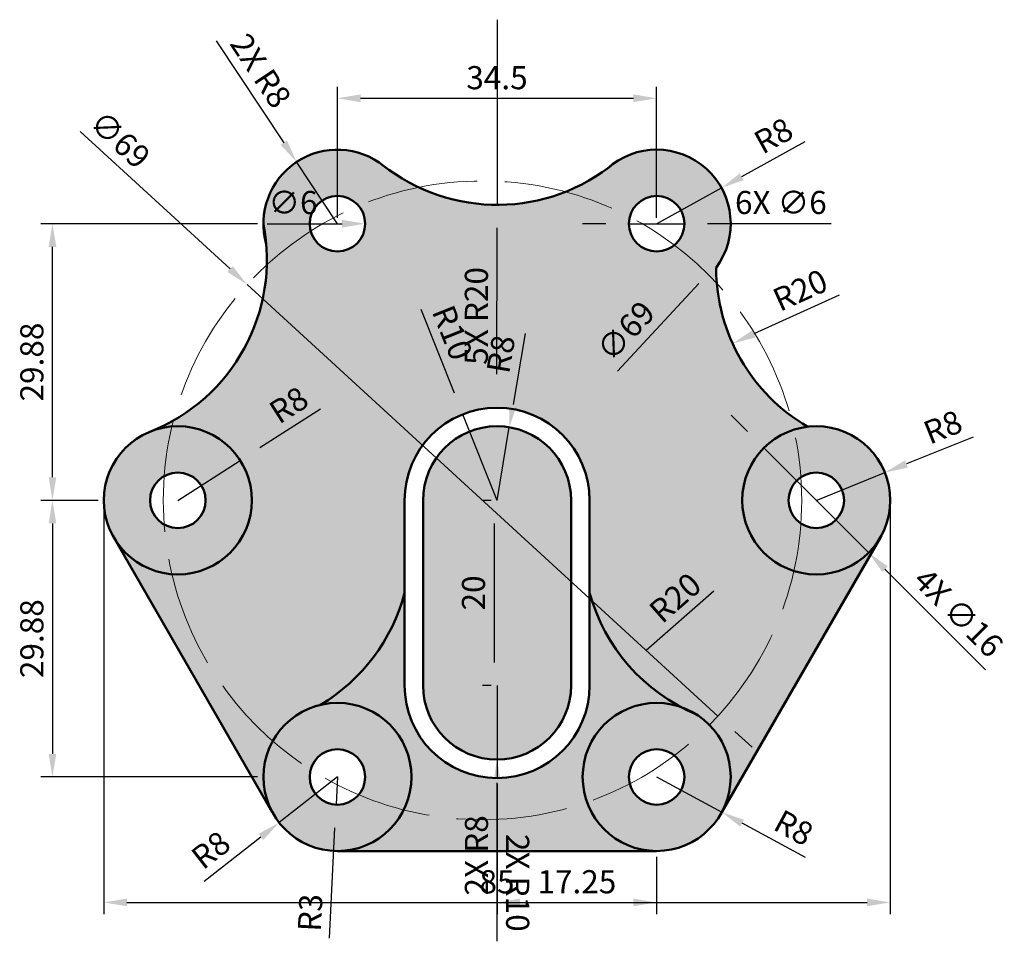
# Model space of a CAD drawing. Units: millimetres. Extents: x 3056 to 3163, y 1664 to 1764.
import ezdxf

# ---------------------------------------------------------------- set-up
doc = ezdxf.new("R2010")
doc.units = ezdxf.units.MM
doc.linetypes.add('ACAD_ISO02W100', pattern=[15, 12, -3])
for name, color, linetype, lineweight in [('M-CONS', 8, 'ACAD_ISO02W100', 18), ('M-DIMS', 2, 'Continuous', 25), ('M-HATC', 252, 'Continuous', 18), ('M-OUTL', 7, 'Continuous', 50)]:
    doc.layers.add(name, color=color, linetype=linetype, lineweight=lineweight)
doc.styles.get("Standard").update_dxf_attribs({"font": 'arial.ttf'})
doc.dimstyles.new('ISO-25', dxfattribs={"dimtxt": 2.5, "dimasz": 2.5, "dimexe": 1.25, "dimexo": 0.625, "dimtad": 1, "dimtxsty": 'Standard', "dimcen": 2.5, "dimadec": 0, "dimazin": 0, "dimtfac": 1, "dimtmove": 0, "dimatfit": 3, "dimfxl": 1, "dimarcsym": 0})

# ---------------------------------------------------------------- blocks, each defined once
blk = doc.blocks.new('*D1')
at = {"layer": 'Defpoints', "color": 0, "transparency": 16777216}
for p in [(3131.59, 1737.12), (3084.57, 1686.62)]:
    blk.add_point(p, dxfattribs=at)
at = {"layer": 'M-DIMS', "color": 0, "lineweight": -2, "transparency": 16777216}
blk.add_line((3121.1, 1725.84), (3129.89, 1735.29), dxfattribs=at)
at = {"layer": 'M-DIMS', "color": 0, "transparency": 16777216}
blk.add_solid([(3129.59, 1735.57), (3130.2, 1735.01), (3131.59, 1737.12)], dxfattribs=at)
at = {"layer": 'M-DIMS', "color": 0, "transparency": 16777216, "insert": (3122.23, 1729.95), "char_height": 2.5, "attachment_point": 5, "rotation": 47.0416}
blk.add_mtext('∅69', dxfattribs=at)
blk = doc.blocks.new('*D2')
at = {"layer": 'Defpoints', "color": 0, "transparency": 16777216}
for p in [(3087.83, 1741.75), (3093.83, 1741.75)]:
    blk.add_point(p, dxfattribs=at)
at = {"layer": 'M-DIMS', "color": 0, "lineweight": -2, "transparency": 16777216}
blk.add_line((3083.23, 1741.75), (3091.33, 1741.75), dxfattribs=at)
at = {"layer": 'M-DIMS', "color": 0, "transparency": 16777216}
blk.add_solid([(3091.33, 1742.17), (3091.33, 1741.33), (3093.83, 1741.75)], dxfattribs=at)
at = {"layer": 'M-DIMS', "color": 0, "transparency": 16777216, "insert": (3086.03, 1743.72), "char_height": 2.5, "attachment_point": 5}
blk.add_mtext('∅6', dxfattribs=at)
blk = doc.blocks.new('*D3')
at = {"layer": 'Defpoints', "color": 0, "transparency": 16777216}
for p in [(3132.34, 1745.62), (3125.33, 1741.75)]:
    blk.add_point(p, dxfattribs=at)
at = {"layer": 'M-DIMS', "color": 0, "lineweight": -2, "transparency": 16777216}
for p, q in [((3141.34, 1750.59), (3134.52, 1746.83)), ((3125.33, 1741.75), (3132.34, 1745.62))]:
    blk.add_line(p, q, dxfattribs=at)
at = {"layer": 'M-DIMS', "color": 0, "transparency": 16777216}
blk.add_solid([(3134.32, 1747.19), (3134.73, 1746.46), (3132.34, 1745.62)], dxfattribs=at)
at = {"layer": 'M-DIMS', "color": 0, "transparency": 16777216, "insert": (3138.11, 1750.98), "char_height": 2.5, "attachment_point": 5, "rotation": 28.9236}
blk.add_mtext('R8', dxfattribs=at)
blk = doc.blocks.new('*D4')
at = {"layer": 'Defpoints', "color": 0, "transparency": 16777216}
for p in [(3151.75, 1737.08), (3133.54, 1728.81)]:
    blk.add_point(p, dxfattribs=at)
at = {"layer": 'M-DIMS', "color": 0, "lineweight": -2, "transparency": 16777216}
blk.add_line((3145.05, 1734.04), (3135.82, 1729.85), dxfattribs=at)
at = {"layer": 'M-DIMS', "color": 0, "transparency": 16777216}
blk.add_solid([(3135.65, 1730.22), (3135.99, 1729.47), (3133.54, 1728.81)], dxfattribs=at)
at = {"layer": 'M-DIMS', "color": 0, "transparency": 16777216, "insert": (3140.98, 1734.28), "char_height": 2.5, "attachment_point": 5, "rotation": 24.4299}
blk.add_mtext('R20', dxfattribs=at)
blk = doc.blocks.new('*D5')
at = {"layer": 'Defpoints', "color": 0, "transparency": 16777216}
for p in [(3109.41, 1719.76), (3108.08, 1711.87)]:
    blk.add_point(p, dxfattribs=at)
at = {"layer": 'M-DIMS', "color": 0, "lineweight": -2, "transparency": 16777216}
for p, q in [((3111.12, 1729.9), (3109.83, 1722.23)), ((3108.08, 1711.87), (3109.41, 1719.76))]:
    blk.add_line(p, q, dxfattribs=at)
at = {"layer": 'M-DIMS', "color": 0, "transparency": 16777216}
blk.add_solid([(3109.42, 1722.29), (3110.24, 1722.16), (3109.41, 1719.76)], dxfattribs=at)
at = {"layer": 'M-DIMS', "color": 0, "transparency": 16777216, "insert": (3108.81, 1727.61), "char_height": 2.5, "attachment_point": 5, "rotation": 80.4313}
blk.add_mtext('R8', dxfattribs=at)
blk = doc.blocks.new('*D6')
at = {"layer": 'Defpoints', "color": 0, "transparency": 16777216}
for p in [(3104.38, 1721.16), (3108.08, 1711.87)]:
    blk.add_point(p, dxfattribs=at)
at = {"layer": 'M-DIMS', "color": 0, "lineweight": -2, "transparency": 16777216}
for p, q in [((3099.86, 1732.51), (3103.45, 1723.48)), ((3108.08, 1711.87), (3104.38, 1721.16))]:
    blk.add_line(p, q, dxfattribs=at)
at = {"layer": 'M-DIMS', "color": 0, "transparency": 16777216}
blk.add_solid([(3103.84, 1723.64), (3103.07, 1723.33), (3104.38, 1721.16)], dxfattribs=at)
at = {"layer": 'M-DIMS', "color": 0, "transparency": 16777216, "insert": (3102.96, 1729.86), "char_height": 2.5, "attachment_point": 5, "rotation": 291.7372}
blk.add_mtext('R10', dxfattribs=at)
blk = doc.blocks.new('*D7')
at = {"layer": 'Defpoints', "color": 0, "transparency": 16777216}
for p in [(3137.36, 1707.2), (3122.33, 1694)]:
    blk.add_point(p, dxfattribs=at)
at = {"layer": 'M-DIMS', "color": 0, "lineweight": -2, "transparency": 16777216}
blk.add_line((3131.51, 1702.06), (3124.21, 1695.65), dxfattribs=at)
at = {"layer": 'M-DIMS', "color": 0, "transparency": 16777216}
blk.add_solid([(3123.93, 1695.97), (3124.48, 1695.34), (3122.33, 1694)], dxfattribs=at)
at = {"layer": 'M-DIMS', "color": 0, "transparency": 16777216, "insert": (3127.55, 1701.11), "char_height": 2.5, "attachment_point": 5, "rotation": 41.2749}
blk.add_mtext('R20', dxfattribs=at)
blk = doc.blocks.new('*D8')
at = {"layer": 'Defpoints', "color": 0, "transparency": 16777216}
for p in [(3090.83, 1681.99), (3090.69, 1679)]:
    blk.add_point(p, dxfattribs=at)
at = {"layer": 'M-DIMS', "color": 0, "lineweight": -2, "transparency": 16777216}
for p, q in [((3090.83, 1681.99), (3090.69, 1679)), ((3089.98, 1664.59), (3090.56, 1676.5))]:
    blk.add_line(p, q, dxfattribs=at)
at = {"layer": 'M-DIMS', "color": 0, "transparency": 16777216}
blk.add_solid([(3090.15, 1676.52), (3090.98, 1676.48), (3090.69, 1679)], dxfattribs=at)
at = {"layer": 'M-DIMS', "color": 0, "transparency": 16777216, "insert": (3088.21, 1667.32), "char_height": 2.5, "attachment_point": 5, "rotation": 87.1851}
blk.add_mtext('R3', dxfattribs=at)
blk = doc.blocks.new('*D9')
at = {"layer": 'Defpoints', "color": 0, "transparency": 16777216}
for p in [(3090.83, 1681.99), (3084.53, 1677.06)]:
    blk.add_point(p, dxfattribs=at)
at = {"layer": 'M-DIMS', "color": 0, "lineweight": -2, "transparency": 16777216}
for p, q in [((3090.83, 1681.99), (3084.53, 1677.06)), ((3076.44, 1670.72), (3082.57, 1675.52))]:
    blk.add_line(p, q, dxfattribs=at)
at = {"layer": 'M-DIMS', "color": 0, "transparency": 16777216}
blk.add_solid([(3082.31, 1675.85), (3082.82, 1675.19), (3084.53, 1677.06)], dxfattribs=at)
at = {"layer": 'M-DIMS', "color": 0, "transparency": 16777216, "insert": (3077.34, 1673.85), "char_height": 2.5, "attachment_point": 5, "rotation": 38.0577}
blk.add_mtext('R8', dxfattribs=at)
blk = doc.blocks.new('*D10')
at = {"layer": 'Defpoints', "color": 0, "transparency": 16777216}
for p in [(3125.33, 1681.99), (3132.37, 1678.19)]:
    blk.add_point(p, dxfattribs=at)
at = {"layer": 'M-DIMS', "color": 0, "lineweight": -2, "transparency": 16777216}
for p, q in [((3125.33, 1681.99), (3132.37, 1678.19)), ((3141.42, 1673.3), (3134.57, 1677))]:
    blk.add_line(p, q, dxfattribs=at)
at = {"layer": 'M-DIMS', "color": 0, "transparency": 16777216}
blk.add_solid([(3134.77, 1677.37), (3134.37, 1676.63), (3132.37, 1678.19)], dxfattribs=at)
at = {"layer": 'M-DIMS', "color": 0, "transparency": 16777216, "insert": (3140, 1676.23), "char_height": 2.5, "attachment_point": 5, "rotation": 331.5993}
blk.add_mtext('R8', dxfattribs=at)
blk = doc.blocks.new('*D11')
at = {"layer": 'Defpoints', "color": 0, "transparency": 16777216}
for p in [(3150, 1714.87), (3142.58, 1711.87)]:
    blk.add_point(p, dxfattribs=at)
at = {"layer": 'M-DIMS', "color": 0, "lineweight": -2, "transparency": 16777216}
for p, q in [((3159.54, 1718.71), (3152.32, 1715.8)), ((3142.58, 1711.87), (3150, 1714.87))]:
    blk.add_line(p, q, dxfattribs=at)
at = {"layer": 'M-DIMS', "color": 0, "transparency": 16777216}
blk.add_solid([(3152.17, 1716.19), (3152.48, 1715.41), (3150, 1714.87)], dxfattribs=at)
at = {"layer": 'M-DIMS', "color": 0, "transparency": 16777216, "insert": (3156.38, 1719.49), "char_height": 2.5, "attachment_point": 5, "rotation": 21.9727}
blk.add_mtext('R8', dxfattribs=at)
blk = doc.blocks.new('*D12')
at = {"layer": 'Defpoints', "color": 0, "transparency": 16777216}
for p in [(3080.33, 1716.18), (3073.58, 1711.87)]:
    blk.add_point(p, dxfattribs=at)
at = {"layer": 'M-DIMS', "color": 0, "lineweight": -2, "transparency": 16777216}
for p, q in [((3088.99, 1721.72), (3082.43, 1717.53)), ((3073.58, 1711.87), (3080.33, 1716.18))]:
    blk.add_line(p, q, dxfattribs=at)
at = {"layer": 'M-DIMS', "color": 0, "transparency": 16777216}
blk.add_solid([(3082.21, 1717.88), (3082.66, 1717.17), (3080.33, 1716.18)], dxfattribs=at)
at = {"layer": 'M-DIMS', "color": 0, "transparency": 16777216, "insert": (3085.74, 1721.9), "char_height": 2.5, "attachment_point": 5, "rotation": 32.5786}
blk.add_mtext('R8', dxfattribs=at)
blk = doc.blocks.new('*D13')
at = {"layer": 'Defpoints', "color": 0, "transparency": 16777216}
for p in [(3108.08, 1711.87), (3107.76, 1691.87), (3108.08, 1691.87)]:
    blk.add_point(p, dxfattribs=at)
at = {"layer": 'M-DIMS', "color": 0, "lineweight": -2, "transparency": 16777216}
for p, q in [((3107.46, 1711.87), (3106.51, 1711.87)), ((3107.76, 1709.37), (3107.76, 1694.37)), ((3107.46, 1691.87), (3106.51, 1691.87))]:
    blk.add_line(p, q, dxfattribs=at)
at = {"layer": 'M-DIMS', "color": 0, "transparency": 16777216}
for points in [[(3107.35, 1709.37), (3108.18, 1709.37), (3107.76, 1711.87)], [(3107.35, 1694.37), (3108.18, 1694.37), (3107.76, 1691.87)]]:
    blk.add_solid(points, dxfattribs=at)
at = {"layer": 'M-DIMS', "color": 0, "transparency": 16777216, "insert": (3105.86, 1701.87), "char_height": 2.5, "attachment_point": 5, "rotation": 90}
blk.add_mtext('20', dxfattribs=at)
blk = doc.blocks.new('MOUNTING-BOSS-16-BORE-6')
for radius in [8, 3]:
    blk.add_circle((8, 8), radius)
blk = doc.blocks.new('*D15')
at = {"layer": 'Defpoints', "color": 0, "transparency": 16777216}
for p in [(3065.58, 1711.87), (3150.58, 1711.87), (3150.58, 1668.44)]:
    blk.add_point(p, dxfattribs=at)
at = {"layer": 'M-DIMS', "color": 0, "lineweight": -2, "transparency": 16777216}
for p, q in [((3065.58, 1711.25), (3065.58, 1667.19)), ((3150.58, 1711.25), (3150.58, 1667.19)), ((3068.08, 1668.44), (3148.08, 1668.44))]:
    blk.add_line(p, q, dxfattribs=at)
at = {"layer": 'M-DIMS', "color": 0, "transparency": 16777216}
for points in [[(3068.08, 1668.86), (3068.08, 1668.03), (3065.58, 1668.44)], [(3148.08, 1668.86), (3148.08, 1668.03), (3150.58, 1668.44)]]:
    blk.add_solid(points, dxfattribs=at)
at = {"layer": 'M-DIMS', "color": 0, "transparency": 16777216, "insert": (3108.08, 1670.35), "char_height": 2.5, "attachment_point": 5}
blk.add_mtext('85', dxfattribs=at)
blk = doc.blocks.new('*D16')
at = {"layer": 'Defpoints', "color": 0, "transparency": 16777216}
for p in [(3125.33, 1755.3), (3090.83, 1741.75), (3125.33, 1741.75)]:
    blk.add_point(p, dxfattribs=at)
at = {"layer": 'M-DIMS', "color": 0, "lineweight": -2, "transparency": 16777216}
for p, q in [((3090.83, 1742.37), (3090.83, 1756.55)), ((3125.33, 1742.37), (3125.33, 1756.55)), ((3093.33, 1755.3), (3122.83, 1755.3))]:
    blk.add_line(p, q, dxfattribs=at)
at = {"layer": 'M-DIMS', "color": 0, "transparency": 16777216}
for points in [[(3093.33, 1755.72), (3093.33, 1754.88), (3090.83, 1755.3)], [(3122.83, 1755.72), (3122.83, 1754.88), (3125.33, 1755.3)]]:
    blk.add_solid(points, dxfattribs=at)
at = {"layer": 'M-DIMS', "color": 0, "transparency": 16777216, "insert": (3108.08, 1757.2), "char_height": 2.5, "attachment_point": 5}
blk.add_mtext('34.5', dxfattribs=at)
blk = doc.blocks.new('*D17')
at = {"layer": 'Defpoints', "color": 0, "transparency": 16777216}
for p in [(3108.08, 1681.87), (3125.33, 1673.99), (3125.33, 1668.44)]:
    blk.add_point(p, dxfattribs=at)
at = {"layer": 'M-DIMS', "color": 0, "lineweight": -2, "transparency": 16777216}
for p, q in [((3108.08, 1681.25), (3108.08, 1667.19)), ((3125.33, 1673.37), (3125.33, 1667.19)), ((3110.58, 1668.44), (3122.83, 1668.44))]:
    blk.add_line(p, q, dxfattribs=at)
at = {"layer": 'M-DIMS', "color": 0, "transparency": 16777216}
for points in [[(3110.58, 1668.86), (3110.58, 1668.03), (3108.08, 1668.44)], [(3122.83, 1668.86), (3122.83, 1668.03), (3125.33, 1668.44)]]:
    blk.add_solid(points, dxfattribs=at)
at = {"layer": 'M-DIMS', "color": 0, "transparency": 16777216, "insert": (3116.71, 1670.35), "char_height": 2.5, "attachment_point": 5}
blk.add_mtext('17.25', dxfattribs=at)
blk = doc.blocks.new('*D18')
at = {"layer": 'Defpoints', "color": 0, "transparency": 16777216}
for p in [(3060.03, 1741.75), (3082.83, 1741.75), (3065.58, 1711.87)]:
    blk.add_point(p, dxfattribs=at)
at = {"layer": 'M-DIMS', "color": 0, "lineweight": -2, "transparency": 16777216}
for p, q in [((3082.21, 1741.75), (3058.78, 1741.75)), ((3060.03, 1714.37), (3060.03, 1739.25)), ((3064.96, 1711.87), (3058.78, 1711.87))]:
    blk.add_line(p, q, dxfattribs=at)
at = {"layer": 'M-DIMS', "color": 0, "transparency": 16777216}
for points in [[(3059.62, 1739.25), (3060.45, 1739.25), (3060.03, 1741.75)], [(3059.62, 1714.37), (3060.45, 1714.37), (3060.03, 1711.87)]]:
    blk.add_solid(points, dxfattribs=at)
at = {"layer": 'M-DIMS', "color": 0, "transparency": 16777216, "insert": (3058.13, 1726.81), "char_height": 2.5, "attachment_point": 5, "rotation": 90}
blk.add_mtext('29.88', dxfattribs=at)
blk = doc.blocks.new('*D19')
at = {"layer": 'Defpoints', "color": 0, "transparency": 16777216}
for p in [(3065.58, 1711.87), (3060.03, 1681.99), (3082.83, 1681.99)]:
    blk.add_point(p, dxfattribs=at)
at = {"layer": 'M-DIMS', "color": 0, "lineweight": -2, "transparency": 16777216}
for p, q in [((3064.96, 1711.87), (3058.78, 1711.87)), ((3060.03, 1709.37), (3060.03, 1684.49)), ((3082.21, 1681.99), (3058.78, 1681.99))]:
    blk.add_line(p, q, dxfattribs=at)
at = {"layer": 'M-DIMS', "color": 0, "transparency": 16777216}
for points in [[(3059.62, 1709.37), (3060.45, 1709.37), (3060.03, 1711.87)], [(3059.62, 1684.49), (3060.45, 1684.49), (3060.03, 1681.99)]]:
    blk.add_solid(points, dxfattribs=at)
at = {"layer": 'M-DIMS', "color": 0, "transparency": 16777216, "insert": (3058.13, 1696.93), "char_height": 2.5, "attachment_point": 5, "rotation": 90}
blk.add_mtext('29.88', dxfattribs=at)
blk = doc.blocks.new('*D20')
at = {"layer": 'Defpoints', "color": 0, "transparency": 16777216}
for p in [(3122.33, 1741.75), (3128.33, 1741.75)]:
    blk.add_point(p, dxfattribs=at)
at = {"layer": 'M-DIMS', "color": 0, "lineweight": -2, "transparency": 16777216}
for p, q in [((3119.83, 1741.75), (3117.33, 1741.75)), ((3122.33, 1741.75), (3128.33, 1741.75)), ((3144.19, 1741.75), (3130.83, 1741.75))]:
    blk.add_line(p, q, dxfattribs=at)
at = {"layer": 'M-DIMS', "color": 0, "transparency": 16777216}
for points in [[(3119.83, 1742.17), (3119.83, 1741.33), (3122.33, 1741.75)], [(3130.83, 1742.17), (3130.83, 1741.33), (3128.33, 1741.75)]]:
    blk.add_solid(points, dxfattribs=at)
at = {"layer": 'M-DIMS', "color": 0, "transparency": 16777216, "insert": (3138.76, 1743.72), "char_height": 2.5, "attachment_point": 5, "rotation": 0.0066}
blk.add_mtext('6X ∅6', dxfattribs=at)
blk = doc.blocks.new('*D21')
at = {"layer": 'Defpoints', "color": 0, "transparency": 16777216}
for p in [(3136.93, 1717.53), (3148.24, 1706.22)]:
    blk.add_point(p, dxfattribs=at)
at = {"layer": 'M-DIMS', "color": 0, "lineweight": -2, "transparency": 16777216}
for p, q in [((3135.16, 1719.3), (3133.39, 1721.06)), ((3136.93, 1717.53), (3148.24, 1706.22)), ((3160.89, 1693.57), (3150.01, 1704.45))]:
    blk.add_line(p, q, dxfattribs=at)
at = {"layer": 'M-DIMS', "color": 0, "transparency": 16777216}
for points in [[(3135.45, 1719.59), (3134.86, 1719), (3136.93, 1717.53)], [(3150.3, 1704.74), (3149.71, 1704.15), (3148.24, 1706.22)]]:
    blk.add_solid(points, dxfattribs=at)
at = {"layer": 'M-DIMS', "color": 0, "transparency": 16777216, "insert": (3157.73, 1699.52), "char_height": 2.5, "attachment_point": 5, "rotation": 315.0013}
blk.add_mtext('4X ∅16', dxfattribs=at)
blk = doc.blocks.new('*D22')
at = {"layer": 'Defpoints', "color": 0, "transparency": 16777216}
for p in [(3081.07, 1735.17), (3131.96, 1688.57)]:
    blk.add_point(p, dxfattribs=at)
at = {"layer": 'M-DIMS', "color": 0, "lineweight": -2, "transparency": 16777216}
for p, q in [((3063.02, 1751.7), (3079.23, 1736.86)), ((3131.96, 1688.57), (3081.07, 1735.17)), ((3133.8, 1686.89), (3135.65, 1685.2))]:
    blk.add_line(p, q, dxfattribs=at)
at = {"layer": 'M-DIMS', "color": 0, "transparency": 16777216}
for points in [[(3079.51, 1737.17), (3078.94, 1736.55), (3081.07, 1735.17)], [(3134.08, 1687.19), (3133.52, 1686.58), (3131.96, 1688.57)]]:
    blk.add_solid(points, dxfattribs=at)
at = {"layer": 'M-DIMS', "color": 0, "transparency": 16777216, "insert": (3067.13, 1750.6), "char_height": 2.5, "attachment_point": 5, "rotation": 317.5212}
blk.add_mtext('∅69', dxfattribs=at)
blk = doc.blocks.new('*D23')
at = {"layer": 'Defpoints', "color": 0, "transparency": 16777216}
for p in [(3108.11, 1763.79), (3108.08, 1743.79)]:
    blk.add_point(p, dxfattribs=at)
at = {"layer": 'M-DIMS', "color": 0, "lineweight": -2, "transparency": 16777216}
for p, q in [((3108.11, 1763.79), (3108.08, 1743.79)), ((3108.06, 1725.49), (3108.08, 1741.29))]:
    blk.add_line(p, q, dxfattribs=at)
at = {"layer": 'M-DIMS', "color": 0, "transparency": 16777216}
blk.add_solid([(3107.66, 1741.29), (3108.5, 1741.29), (3108.08, 1743.79)], dxfattribs=at)
at = {"layer": 'M-DIMS', "color": 0, "transparency": 16777216, "insert": (3106.17, 1731.79), "char_height": 2.5, "attachment_point": 5, "rotation": 89.9384}
blk.add_mtext('5X R20', dxfattribs=at)
blk = doc.blocks.new('*D24')
at = {"layer": 'Defpoints', "color": 0, "transparency": 16777216}
for p in [(3108.08, 1691.87), (3108.08, 1681.87)]:
    blk.add_point(p, dxfattribs=at)
at = {"layer": 'M-DIMS', "color": 0, "lineweight": -2, "transparency": 16777216}
for p, q in [((3108.08, 1691.87), (3108.08, 1681.87)), ((3108.08, 1664.24), (3108.08, 1679.37))]:
    blk.add_line(p, q, dxfattribs=at)
at = {"layer": 'M-DIMS', "color": 0, "transparency": 16777216}
blk.add_solid([(3108.5, 1679.37), (3107.67, 1679.37), (3108.08, 1681.87)], dxfattribs=at)
at = {"layer": 'M-DIMS', "color": 0, "transparency": 16777216, "insert": (3109.99, 1670.56), "char_height": 2.5, "attachment_point": 5, "rotation": 270.0002}
blk.add_mtext('2X R10', dxfattribs=at)
blk = doc.blocks.new('*D25')
at = {"layer": 'Defpoints', "color": 0, "transparency": 16777216}
for p in [(3086.42, 1748.42), (3090.83, 1741.75)]:
    blk.add_point(p, dxfattribs=at)
at = {"layer": 'M-DIMS', "color": 0, "lineweight": -2, "transparency": 16777216}
for p, q in [((3077.74, 1761.51), (3085.03, 1750.5)), ((3090.83, 1741.75), (3086.42, 1748.42))]:
    blk.add_line(p, q, dxfattribs=at)
at = {"layer": 'M-DIMS', "color": 0, "transparency": 16777216}
blk.add_solid([(3085.38, 1750.73), (3084.69, 1750.27), (3086.42, 1748.42)], dxfattribs=at)
at = {"layer": 'M-DIMS', "color": 0, "transparency": 16777216, "insert": (3082.28, 1758.1), "char_height": 2.5, "attachment_point": 5, "rotation": 303.5276}
blk.add_mtext('2X R8', dxfattribs=at)
blk = doc.blocks.new('*D26')
at = {"layer": 'Defpoints', "color": 0, "transparency": 16777216}
for p in [(3108.08, 1691.87), (3108.08, 1683.87)]:
    blk.add_point(p, dxfattribs=at)
at = {"layer": 'M-DIMS', "color": 0, "lineweight": -2, "transparency": 16777216}
for p, q in [((3108.08, 1691.87), (3108.08, 1683.87)), ((3108.08, 1668.17), (3108.08, 1681.37))]:
    blk.add_line(p, q, dxfattribs=at)
at = {"layer": 'M-DIMS', "color": 0, "transparency": 16777216}
blk.add_solid([(3107.67, 1681.37), (3108.5, 1681.37), (3108.08, 1683.87)], dxfattribs=at)
at = {"layer": 'M-DIMS', "color": 0, "transparency": 16777216, "insert": (3106.18, 1673.52), "char_height": 2.5, "attachment_point": 5, "rotation": 90}
blk.add_mtext('2X R8', dxfattribs=at)

msp = doc.modelspace()

# ---------------------------------------------------------------- hatches: boundary and pattern name
at = {"layer": 'M-HATC'}
h = msp.add_hatch(color=256, dxfattribs=at)
h.set_gradient(color1=(255, 255, 255), color2=(0, 255, 255), tint=1, name='INVSPHERICAL')
h.paths.add_polyline_path([(3131.752, 1736.973, 0.8439134), (3120.862, 1748.383, -0.3543215), (3095.679, 1748.115, 0.6204861), (3082.834, 1741.75, -0.3599737), (3070.694, 1719.331, -0.5271202), (3081.584, 1711.872, -0.7672909), (3066.656, 1707.871), (3083.797, 1678.189, -0.1245598), (3082.834, 1681.994, -0.3481695), (3089.005, 1689.782, 0.1962669), (3098.084, 1701.872), (3098.084, 1711.872, -1), (3118.084, 1711.872), (3118.084, 1701.872, 0.2053969), (3127.933, 1689.56, -0.3203024), (3133.334, 1681.994, -0.1245598), (3132.371, 1678.189), (3149.512, 1707.871, -0.7672909), (3134.584, 1711.872, -0.3805737), (3141.656, 1719.818, -0.265009)])
h.paths.add_polyline_path([(3087.834, 1741.75, -1), (3093.834, 1741.75, -1)], flags=16)
h.paths.add_polyline_path([(3122.334, 1741.75, -1), (3128.334, 1741.75, -1)], flags=16)
h.paths.add_polyline_path([(3121.467, 1725.306), (3126.817, 1731.051), (3123.047, 1734.562), (3117.696, 1728.816)], flags=24)
h.paths.add_polyline_path([(3083.085, 1741.11), (3088.994, 1741.11), (3088.994, 1746.262), (3083.085, 1746.262)], flags=24)
h.paths.add_polyline_path([(3110.887, 1724.304), (3111.837, 1729.939), (3106.757, 1730.796), (3105.807, 1725.161)], flags=24)
h.paths.add_polyline_path([(3099.107, 1732.504), (3101.943, 1725.392), (3106.728, 1727.3), (3103.892, 1734.412)], flags=24)
h.paths.add_polyline_path([(3126.342, 1696.598), (3132.097, 1701.649), (3128.698, 1705.52), (3122.944, 1700.469)], flags=24)
h.paths.add_polyline_path([(3084.683, 1718.136), (3089.498, 1721.213), (3086.724, 1725.554), (3081.909, 1722.477)], flags=24)
h = msp.add_hatch(color=256, dxfattribs=at)
h.set_gradient(color1=(255, 255, 255), color2=(248, 215, 49), tint=1, name='INVSPHERICAL')
h.paths.add_polyline_path([(3070.694, 1719.331, -0.0019683), (3070.548, 1719.273, 0.3042702), (3065.584, 1711.872, 1), (3081.584, 1711.872, 0.5271202)])
h.paths.add_polyline_path([(3076.584, 1711.872, -1), (3070.584, 1711.872, -1)], flags=16)
h.paths.add_polyline_path([(3082.834, 1681.994, 1), (3098.834, 1681.994, 1)])
h.paths.add_polyline_path([(3093.834, 1681.994, -1), (3087.834, 1681.994, -1)], flags=16)
h.paths.add_polyline_path([(3129.581, 1688.774, -0.0228354), (3127.933, 1689.56, 0.5148044), (3117.334, 1681.994, 1), (3133.334, 1681.994, 0.25832)])
h.paths.add_polyline_path([(3128.334, 1681.994, -1), (3122.334, 1681.994, -1)], flags=16)
h.paths.add_polyline_path([(3134.584, 1711.872, 1), (3150.584, 1711.872, 1)])
h.paths.add_polyline_path([(3145.584, 1711.872, -1), (3139.584, 1711.872, -1)], flags=16)
h = msp.add_hatch(color=256, dxfattribs=at)
h.set_gradient(color1=(255, 255, 255), color2=(255, 0, 255), tint=1, name='INVCYLINDER')
h.paths.add_polyline_path([(3100.084, 1711.872), (3100.084, 1691.872, 1), (3116.084, 1691.872), (3116.084, 1711.872, 1)])
h.paths.add_polyline_path([(3108.462, 1699.337), (3108.462, 1704.472), (3103.31, 1704.472), (3103.31, 1699.337)], flags=24)
h = msp.add_hatch(color=256, dxfattribs=at)
h.set_gradient(color1=(255, 255, 255), color2=(88, 186, 72), tint=1, name='HEMISPHERICAL')
h.paths.add_polyline_path([(3117.334, 1681.994, -0.5148044), (3127.933, 1689.56, -0.2053969), (3118.084, 1701.872), (3118.084, 1691.872, -1), (3098.084, 1691.872), (3098.084, 1701.872, -0.1962669), (3089.005, 1689.782, -0.483493), (3098.834, 1681.994, -0.4142136), (3090.834, 1673.994), (3125.334, 1673.994, -0.4142136)])

# ---------------------------------------------------------------- linework, layer by layer
at = {"layer": 'M-CONS'}
msp.add_circle((3106.514, 1711.872), 34.5, dxfattribs=at)
at = {"layer": 'M-OUTL'}
for p, q in [((3098.084, 1711.872), (3098.084, 1691.872)), ((3100.084, 1711.872), (3100.084, 1691.872)), ((3116.084, 1711.872), (3116.084, 1691.872)), ((3118.084, 1711.872), (3118.084, 1691.872)), ((3083.797, 1678.189), (3066.656, 1707.871)), ((3132.371, 1678.189), (3149.512, 1707.871)), ((3090.834, 1673.994), (3125.334, 1673.994))]:
    msp.add_line(p, q, dxfattribs=at)
for centre in [(3090.834, 1741.75), (3125.334, 1741.75)]:
    msp.add_circle(centre, 3, dxfattribs=at)
for centre, radius, start, end in [((3090.834, 1741.75), 8, 51.10088, 195.95248), ((3125.334, 1741.75), 8, 323.34204, 132.04836), ((3108.106, 1763.787), 20, 231.58779, 309.62911), ((3063.212, 1737.879), 20, 291.51682, 11.15807), ((3151.751, 1737.083), 20, 180.31458, 239.68542), ((3108.084, 1711.872), 10, 0, 180), ((3108.084, 1711.872), 8, 0, 180), ((3078.738, 1706.946), 20, 300.88726, 345.30374), ((3137.362, 1707.198), 20, 195.44474, 247.10511), ((3108.084, 1691.872), 10, 180, 0), ((3108.084, 1691.872), 8, 180, 0)]:
    msp.add_arc(centre, radius, start, end, dxfattribs=at)

# ---------------------------------------------------------------- block references
for p in [(3065.584, 1703.872), (3134.584, 1703.872), (3082.834, 1673.994), (3117.334, 1673.994)]:
    msp.add_blockref('MOUNTING-BOSS-16-BORE-6', p, dxfattribs=at)

# ---------------------------------------------------------------- dimensions: what is measured, and where the dimension line sits
at = {"layer": 'M-DIMS'}
dim = msp.add_radius_dim(center=(3108.106, 1763.787), mpoint=(3108.084, 1743.787), text='5X <>', dimstyle='ISO-25', override={"dimdec": 0, "dimlfac": 1, "dimrnd": 0, "dimzin": 0, "dimdsep": 46, "dimlunit": 2}, dxfattribs=at)
dim.commit()
dim.dimension.update_dxf_attribs({"geometry": '*D23', "text_midpoint": (3108.071, 1731.787), "dimtype": 164})
for center, mpoint, picture, middle in [((3090.834, 1741.75), (3086.415, 1748.419), '*D25', (3082.283, 1758.097)), ((3108.084, 1691.872), (3108.084, 1683.872), '*D26', (3106.183, 1673.521)), ((3108.084, 1691.872), (3108.084, 1681.872), '*D24', (3109.985, 1670.557))]:
    dim = msp.add_radius_dim(center=center, mpoint=mpoint, text='2X <>', dimstyle='ISO-25', override={"dimdec": 0, "dimlfac": 1, "dimrnd": 0, "dimzin": 0, "dimdsep": 46, "dimlunit": 2}, dxfattribs=at)
    dim.commit()
    dim.dimension.update_dxf_attribs({"geometry": picture, "text_midpoint": middle})
for base, p1, p2, override, picture, middle in [((3125.334, 1755.3), (3090.834, 1741.75), (3125.334, 1741.75), {"dimdec": 1, "dimlfac": 1, "dimrnd": 0, "dimzin": 0, "dimdsep": 46, "dimlunit": 2}, '*D16', (3108.084, 1757.202)), ((3150.584, 1668.444), (3065.584, 1711.872), (3150.584, 1711.872), {"dimdec": 0, "dimlfac": 1, "dimrnd": 0, "dimzin": 0, "dimdsep": 46, "dimlunit": 2}, '*D15', (3108.084, 1670.345)), ((3125.334, 1668.444), (3108.084, 1681.872), (3125.334, 1673.994), {"dimdec": 2, "dimlfac": 1, "dimrnd": 0, "dimzin": 0, "dimdsep": 46, "dimlunit": 2}, '*D17', (3116.709, 1670.345))]:
    dim = msp.add_linear_dim(base=base, p1=p1, p2=p2, dimstyle='ISO-25', override=override, dxfattribs=at)
    dim.commit()
    dim.dimension.update_dxf_attribs({"geometry": picture, "text_midpoint": middle})
for p1, p2, override, picture, middle in [((3131.959, 1688.573), (3081.07, 1735.17), {"dimdec": 0, "dimlfac": 1, "dimrnd": 0, "dimzin": 0, "dimdsep": 46, "dimlunit": 2}, '*D22', (3065.803, 1749.149)), ((3087.834, 1741.75), (3093.834, 1741.75), {"dimclrd": 0, "dimclre": 0, "dimclrt": 0}, '*D2', (3086.03, 1741.75)), ((3084.573, 1686.623), (3131.595, 1737.121), {"dimclrd": 0, "dimclre": 0, "dimclrt": 0}, '*D1', (3123.67, 1728.61))]:
    dim = msp.add_diameter_dim_2p(p1=p1, p2=p2, dimstyle='ISO-25', override=override, dxfattribs=at)
    dim.commit()
    dim.dimension.update_dxf_attribs({"geometry": picture, "text_midpoint": middle, "dimtype": 163})
for center, mpoint, picture, middle in [((3125.334, 1741.75), (3132.336, 1745.619), '*D3', (3138.106, 1750.98)), ((3108.084, 1711.872), (3104.38, 1721.161), '*D6', (3102.959, 1729.86)), ((3108.084, 1711.872), (3109.414, 1719.76), '*D5', (3108.809, 1727.613)), ((3073.584, 1711.872), (3080.325, 1716.179), '*D12', (3085.742, 1721.897)), ((3142.584, 1711.872), (3150.003, 1714.865), '*D11', (3156.379, 1719.488)), ((3090.834, 1681.994), (3084.535, 1677.062), '*D9', (3077.344, 1673.848)), ((3125.334, 1681.994), (3132.371, 1678.189), '*D10', (3139.999, 1676.226))]:
    dim = msp.add_radius_dim(center=center, mpoint=mpoint, dimstyle='ISO-25', override={"dimclrd": 0, "dimclre": 0, "dimclrt": 0}, dxfattribs=at)
    dim.commit()
    dim.dimension.update_dxf_attribs({"geometry": picture, "text_midpoint": middle})
for p1, p2, text, picture, middle in [((3122.334, 1741.749), (3128.334, 1741.75), '6X <>', '*D20', (3138.764, 1741.751)), ((3136.927, 1717.529), (3148.241, 1706.215), '4X <>', '*D21', (3156.334, 1698.123))]:
    dim = msp.add_diameter_dim_2p(p1=p1, p2=p2, text=text, dimstyle='ISO-25', override={"dimdec": 0, "dimlfac": 1, "dimrnd": 0, "dimzin": 0, "dimdsep": 46, "dimlunit": 2}, dxfattribs=at)
    dim.commit()
    dim.dimension.update_dxf_attribs({"geometry": picture, "text_midpoint": middle})
for base, p1, p2, override, picture, middle in [((3060.034, 1741.75), (3065.584, 1711.872), (3082.834, 1741.75), {"dimdec": 2, "dimlfac": 1, "dimrnd": 0, "dimzin": 0, "dimdsep": 46, "dimlunit": 2}, '*D18', (3058.133, 1726.811)), ((3060.034, 1681.994), (3065.584, 1711.872), (3082.834, 1681.994), {"dimdec": 2, "dimlfac": 1, "dimrnd": 0, "dimzin": 0, "dimdsep": 46, "dimlunit": 2}, '*D19', (3058.133, 1696.933)), ((3107.764, 1691.872), (3108.084, 1711.872), (3108.084, 1691.872), {"dimclrd": 0, "dimclre": 0, "dimclrt": 0}, '*D13', (3105.863, 1701.872))]:
    dim = msp.add_linear_dim(base=base, p1=p1, p2=p2, angle=90, dimstyle='ISO-25', override=override, dxfattribs=at)
    dim.commit()
    dim.dimension.update_dxf_attribs({"geometry": picture, "text_midpoint": middle})
for center, mpoint, picture, middle in [((3151.751, 1737.083), (3133.542, 1728.812), '*D4', (3141.764, 1732.546)), ((3137.362, 1707.198), (3122.331, 1694.004), '*D7', (3128.8, 1699.683)), ((3090.834, 1681.994), (3090.687, 1678.998), '*D8', (3090.108, 1667.23))]:
    dim = msp.add_radius_dim(center=center, mpoint=mpoint, dimstyle='ISO-25', override={"dimclrd": 0, "dimclre": 0, "dimclrt": 0}, dxfattribs=at)
    dim.commit()
    dim.dimension.update_dxf_attribs({"geometry": picture, "text_midpoint": middle, "dimtype": 164})

doc.saveas('drawing.dxf')
